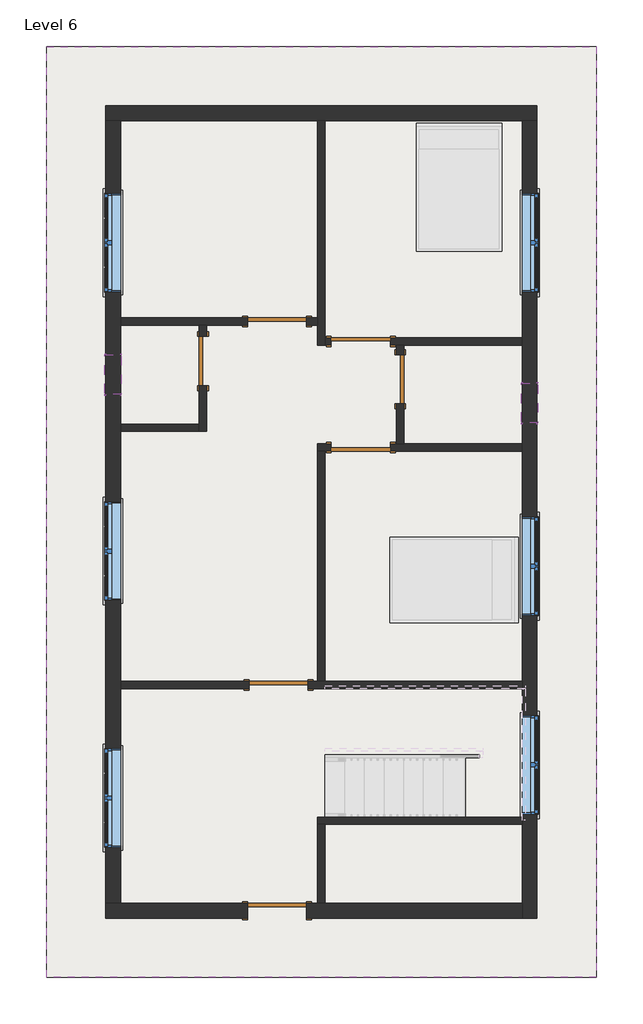
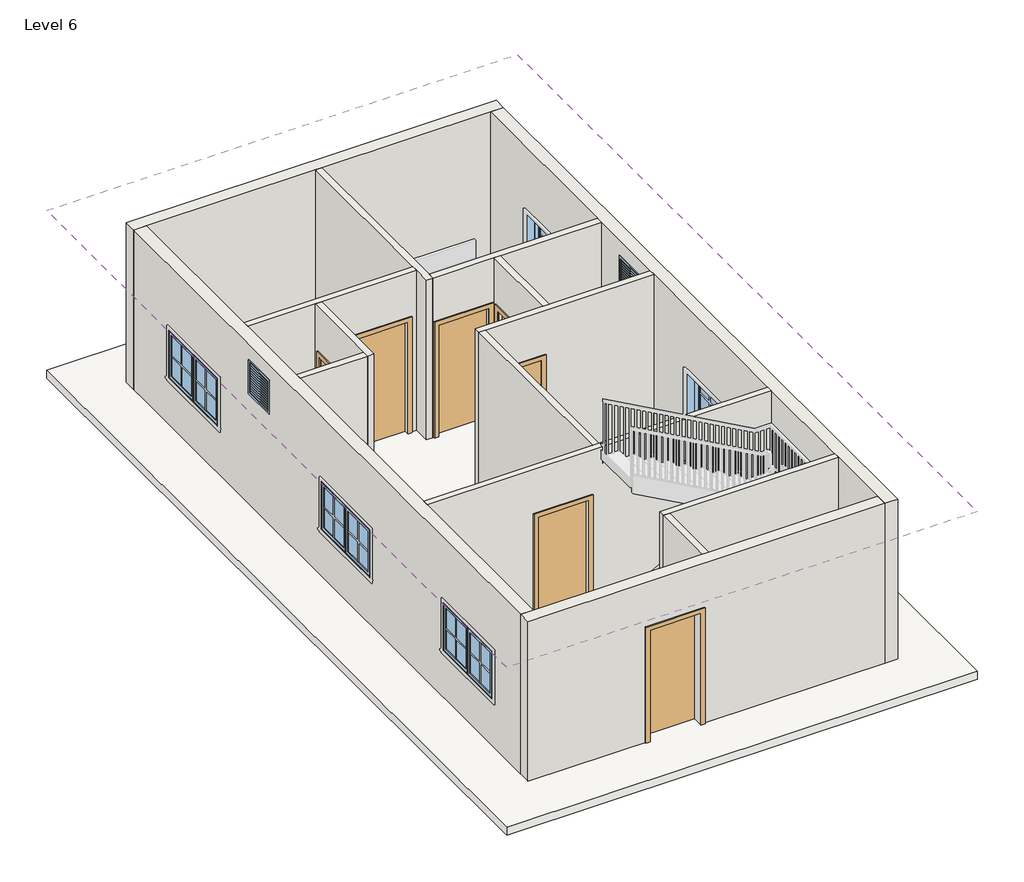
# One storey, part 1 of 3: 15 walls, 8 windows, 7 doors, 2 roofs.
"""IFC4 building model written with IfcOpenShell, lengths in millimetres."""

from ifc_helpers import new_model, si_unit, frame, origin, place, context, project, spatial, polyline, outline, extrude, faceted_brep, transform, mapped, element, save
from components import door_78caadf7, door_214872d5, single_flush_door_3_e5f9f3c4, single_flush_door_3_305aa2a5, single_flush_door_3_0ca8825f, window_casement_double_win_5_c1d95f0f, window_f2d8fef0

model = new_model("IFC4")

# Units and contexts
model_context = context("Model", 3, world=origin())
ifc_project = project(units=[si_unit("LENGTHUNIT", "METRE", prefix="MILLI")], contexts=[model_context])

# Site, building, storey
site = spatial("IfcSite", under=ifc_project)
building = spatial("IfcBuilding", under=site)
storey = spatial("IfcBuildingStorey", under=building, Name="Level 6", Elevation=15849.6)

# Doors
placement = place(None, origin())
door_shape = door_78caadf7(model_context)
element("IfcDoor", 1, ObjectType="Single-Flush : 2'6\"", at=placement, inside=storey, context=model_context, shape_type="MappedRepresentation", body=[
    mapped(door_shape, transform((-35.92188, 1946.24131, 15849.6), x_axis=(0.0, 1.0, 0.0), y_axis=(-1.0, 0.0, 0.0), z_axis=(0.0, 0.0, 1.0))),
])
door_2_shape = door_214872d5(model_context)
element("IfcDoor", 2, ObjectType="Single-Flush : 2'6\"", at=placement, inside=storey, context=model_context, shape_type="MappedRepresentation", body=[
    mapped(door_2_shape, transform((-3083.92188, 2225.64131, 15849.6), x_axis=(0.0, 1.0, 0.0), y_axis=(-1.0, 0.0, 0.0), z_axis=(0.0, 0.0, 1.0))),
])
single_flush_door_3_shape = single_flush_door_3_e5f9f3c4(model_context)
element("IfcDoor", 3, ObjectType="Single-Flush : DOOR 3'", at=placement, inside=storey, context=model_context, shape_type="MappedRepresentation", body=[
    mapped(single_flush_door_3_shape, transform((-1940.92188, 2835.24131, 15849.6), x_axis=(1.0, 0.0, 0.0), y_axis=(0.0, 1.0, 0.0), z_axis=(0.0, 0.0, 1.0))),
])
element("IfcDoor", 4, ObjectType="Single-Flush : DOOR 3'", at=placement, inside=storey, context=model_context, shape_type="MappedRepresentation", body=[
    mapped(single_flush_door_3_shape, transform((-645.52188, 892.14131, 15849.6), x_axis=(-1.0, 0.0, 0.0), y_axis=(0.0, -1.0, 0.0), z_axis=(0.0, 0.0, 1.0))),
])
element("IfcDoor", 5, ObjectType="Single-Flush : DOOR 3'", at=placement, inside=storey, context=model_context, shape_type="MappedRepresentation", body=[
    mapped(single_flush_door_3_shape, transform((-1915.52188, -2778.15869, 15849.6), x_axis=(1.0, 0.0, 0.0), y_axis=(0.0, 1.0, 0.0), z_axis=(0.0, 0.0, 1.0))),
])
single_flush_door_3_2_shape = single_flush_door_3_305aa2a5(model_context)
element("IfcDoor", 6, ObjectType="Single-Flush : DOOR 3'", at=placement, inside=storey, context=model_context, shape_type="MappedRepresentation", body=[
    mapped(single_flush_door_3_2_shape, transform((-645.52188, 2530.44131, 15849.6), x_axis=(-1.0, 0.0, 0.0), y_axis=(0.0, -1.0, 0.0), z_axis=(0.0, 0.0, 1.0))),
])
single_flush_door_3_3_shape = single_flush_door_3_0ca8825f(model_context)
element("IfcDoor", 7, ObjectType="Single-Flush : DOOR 3'", at=placement, inside=storey, context=model_context, shape_type="MappedRepresentation", body=[
    mapped(single_flush_door_3_3_shape, transform((-1940.92188, -6264.30869, 15849.6), x_axis=(1.0, 0.0, 0.0), y_axis=(0.0, 1.0, 0.0), z_axis=(0.0, 0.0, 1.0))),
])

# Roofs
element("IfcRoof", 8, ObjectType="ROOF 6\"", at=placement, inside=storey, context=model_context, shape_type="SweptSolid", body=[
    extrude(outline(polyline([(-5503.27188, 7083.39131), (2993.02812, 7083.39131), (2993.02812, -7293.00869), (-5503.27188, -7293.00869), (-5503.27188, 7083.39131)])), frame((0.0, 0.0, 15697.2), z_axis=(0.0, 0.0, 1.0), x_axis=(1.0, 0.0, 0.0)), (0.0, 0.0, 1.0), 152.4),
])
element("IfcRoof", 9, ObjectType="ROOF 6\"", at=placement, inside=storey, context=model_context, shape_type="SweptSolid", body=[
    extrude(outline(polyline([(-5503.27188, 7083.39131), (2993.02812, 7083.39131), (2993.02812, -7293.00869), (-5503.27188, -7293.00869), (-5503.27188, 7083.39131)])), frame((0.0, 0.0, 18897.6), z_axis=(0.0, 0.0, 1.0), x_axis=(1.0, 0.0, 0.0)), (0.0, 0.0, 1.0), 152.4),
])

# Walls
element("IfcWall", 10, ObjectType="WALL 4.5'", at=placement, inside=storey, context=model_context, shape_type="Brep", body=[
    faceted_brep([(-1312.27188, 5940.39131, 15849.6), (-1312.27188, 2892.39131, 15849.6), (-1312.27188, 2778.09131, 15849.6), (-1312.27188, 2473.29131, 15849.6), (-1312.27188, 2473.29131, 18897.6), (-1312.27188, 2778.09131, 18897.6), (-1312.27188, 2892.39131, 18897.6), (-1312.27188, 5940.39131, 18897.6), (-1197.97188, 5940.39131, 15849.6), (-1197.97188, 5940.39131, 18897.6), (-1197.97188, 2587.59131, 18897.6), (-1197.97188, 2473.29131, 18897.6), (-1197.97188, 2473.29131, 15849.6), (-1197.97188, 2587.59131, 15849.6)], [[[0, 1, 2, 3, 4, 5, 6, 7]], [[8, 9, 10, 11, 12, 13]], [[3, 2, 1, 0, 8, 13, 12]], [[0, 7, 9, 8]], [[4, 3, 12, 11]], [[7, 6, 5, 4, 11, 10, 9]]]),
])
element("IfcWall", 11, ObjectType="WALL 4.5'", at=placement, inside=storey, context=model_context, shape_type="Brep", body=[
    faceted_brep([(-1197.97188, 2473.29131, 15849.6), (-1102.72188, 2473.29131, 15849.6), (-1102.72188, 2473.29131, 17983.2), (-188.32188, 2473.29131, 17983.2), (-188.32188, 2473.29131, 15849.6), (-93.07188, 2473.29131, 15849.6), (21.22812, 2473.29131, 15849.6), (1850.02812, 2473.29131, 15849.6), (1850.02812, 2473.29131, 18897.6), (21.22812, 2473.29131, 18897.6), (-93.07188, 2473.29131, 18897.6), (-1197.97188, 2473.29131, 18897.6), (-1102.72188, 2587.59131, 17983.2), (-1102.72188, 2587.59131, 15849.6), (-1197.97188, 2587.59131, 15849.6), (-1197.97188, 2587.59131, 18897.6), (1850.02812, 2587.59131, 18897.6), (1850.02812, 2587.59131, 15849.6), (-188.32188, 2587.59131, 15849.6), (-188.32188, 2587.59131, 17983.2)], [[[0, 1, 2, 3, 4, 5, 6, 7, 8, 9, 10, 11]], [[12, 13, 14, 15, 16, 17, 18, 19]], [[18, 17, 7, 6, 5, 4]], [[14, 13, 1, 0]], [[0, 11, 15, 14]], [[8, 7, 17, 16]], [[2, 1, 13, 12]], [[3, 2, 12, 19]], [[4, 3, 19, 18]], [[11, 10, 9, 8, 16, 15]]]),
])
element("IfcWall", 12, ObjectType="WALL 4.5'", at=placement, inside=storey, context=model_context, shape_type="Brep", body=[
    faceted_brep([(-1312.27188, 2892.39131, 15849.6), (-1483.72188, 2892.39131, 15849.6), (-1483.72188, 2892.39131, 17983.2), (-2398.12188, 2892.39131, 17983.2), (-2398.12188, 2892.39131, 15849.6), (-4360.27188, 2892.39131, 15849.6), (-4360.27188, 2892.39131, 18897.6), (-1312.27188, 2892.39131, 18897.6), (-1483.72188, 2778.09131, 17983.2), (-1483.72188, 2778.09131, 15849.6), (-1312.27188, 2778.09131, 15849.6), (-1312.27188, 2778.09131, 18897.6), (-3026.77188, 2778.09131, 18897.6), (-3141.07188, 2778.09131, 18897.6), (-4360.27188, 2778.09131, 18897.6), (-4360.27188, 2778.09131, 15849.6), (-3141.07188, 2778.09131, 15849.6), (-3026.77188, 2778.09131, 15849.6), (-2398.12188, 2778.09131, 15849.6), (-2398.12188, 2778.09131, 17983.2)], [[[0, 1, 2, 3, 4, 5, 6, 7]], [[8, 9, 10, 11, 12, 13, 14, 15, 16, 17, 18, 19]], [[10, 9, 1, 0]], [[18, 17, 16, 15, 5, 4]], [[6, 5, 15, 14]], [[0, 7, 11, 10]], [[2, 1, 9, 8]], [[3, 2, 8, 19]], [[4, 3, 19, 18]], [[7, 6, 14, 13, 12, 11]]]),
])
element("IfcWall", 13, ObjectType="WALL 4.5'", at=placement, inside=storey, context=model_context, shape_type="Brep", body=[
    faceted_brep([(-3141.07188, 2778.09131, 15849.6), (-3141.07188, 2606.64131, 15849.6), (-3141.07188, 2606.64131, 17983.2), (-3141.07188, 1844.64131, 17983.2), (-3141.07188, 1844.64131, 15849.6), (-3141.07188, 1254.09131, 15849.6), (-3141.07188, 1139.79131, 15849.6), (-3141.07188, 1139.79131, 18897.6), (-3141.07188, 1254.09131, 18897.6), (-3141.07188, 2778.09131, 18897.6), (-3026.77188, 2606.64131, 17983.2), (-3026.77188, 2606.64131, 15849.6), (-3026.77188, 2778.09131, 15849.6), (-3026.77188, 2778.09131, 18897.6), (-3026.77188, 1139.79131, 18897.6), (-3026.77188, 1139.79131, 15849.6), (-3026.77188, 1844.64131, 15849.6), (-3026.77188, 1844.64131, 17983.2)], [[[0, 1, 2, 3, 4, 5, 6, 7, 8, 9]], [[10, 11, 12, 13, 14, 15, 16, 17]], [[16, 15, 6, 5, 4]], [[12, 11, 1, 0]], [[0, 9, 13, 12]], [[7, 6, 15, 14]], [[2, 1, 11, 10]], [[3, 2, 10, 17]], [[4, 3, 17, 16]], [[9, 8, 7, 14, 13]]]),
])
element("IfcWall", 14, ObjectType="WALL 4.5'", at=placement, inside=storey, context=model_context, shape_type="SweptSolid", body=[
    extrude(outline(polyline([(-4360.27188, 1254.09131), (-3141.07188, 1254.09131), (-3141.07188, 1139.79131), (-4360.27188, 1139.79131), (-4360.27188, 1254.09131)])), frame((0.0, 0.0, 15849.6), z_axis=(0.0, 0.0, 1.0), x_axis=(1.0, 0.0, 0.0)), (0.0, 0.0, 1.0), 3048.0),
])
element("IfcWall", 15, ObjectType="WALL 4.5'", at=placement, inside=storey, context=model_context, shape_type="SweptSolid", body=[
    extrude(outline(polyline([(2473.29131, 15849.6), (2327.24131, 15849.6), (2327.24131, 17983.2), (1565.24131, 17983.2), (1565.24131, 15849.6), (949.29131, 15849.6), (949.29131, 18897.6), (2473.29131, 18897.6), (2473.29131, 15849.6)])), frame((-93.07188, 0.0, 0.0), z_axis=(1.0, 0.0, 0.0), x_axis=(0.0, 1.0, 0.0)), (0.0, 0.0, 1.0), 114.3),
])
element("IfcWall", 16, ObjectType="WALL 4.5'", at=placement, inside=storey, context=model_context, shape_type="Brep", body=[
    faceted_brep([(-1102.72188, 949.29131, 17983.2), (-1102.72188, 949.29131, 15849.6), (-1312.27188, 949.29131, 15849.6), (-1312.27188, 949.29131, 18897.6), (-93.07188, 949.29131, 18897.6), (21.22812, 949.29131, 18897.6), (1850.02812, 949.29131, 18897.6), (1850.02812, 949.29131, 15849.6), (21.22812, 949.29131, 15849.6), (-93.07188, 949.29131, 15849.6), (-188.32188, 949.29131, 15849.6), (-188.32188, 949.29131, 17983.2), (-1312.27188, 834.99131, 15849.6), (-1197.97188, 834.99131, 15849.6), (-1102.72188, 834.99131, 15849.6), (-1102.72188, 834.99131, 17983.2), (-188.32188, 834.99131, 17983.2), (-188.32188, 834.99131, 15849.6), (1850.02812, 834.99131, 15849.6), (1850.02812, 834.99131, 18897.6), (-1197.97188, 834.99131, 18897.6), (-1312.27188, 834.99131, 18897.6)], [[[0, 1, 2, 3, 4, 5, 6, 7, 8, 9, 10, 11]], [[12, 13, 14, 15, 16, 17, 18, 19, 20, 21]], [[2, 1, 14, 13, 12]], [[10, 9, 8, 7, 18, 17]], [[7, 6, 19, 18]], [[3, 2, 12, 21]], [[15, 14, 1, 0]], [[16, 15, 0, 11]], [[17, 16, 11, 10]], [[6, 5, 4, 3, 21, 20, 19]]]),
])
element("IfcWall", 17, ObjectType="WALL 4.5'", at=placement, inside=storey, context=model_context, shape_type="SweptSolid", body=[
    extrude(outline(polyline([(-1312.27188, -2721.00869), (-1312.27188, 834.99131), (-1197.97188, 834.99131), (-1197.97188, -2721.00869), (-1312.27188, -2721.00869)])), frame((0.0, 0.0, 15849.6), z_axis=(0.0, 0.0, 1.0), x_axis=(1.0, 0.0, 0.0)), (0.0, 0.0, 1.0), 3048.0),
])
element("IfcWall", 18, ObjectType="WALL 4.5'", at=placement, inside=storey, context=model_context, shape_type="Brep", body=[
    faceted_brep([(1850.02812, -2721.00869, 15849.6), (-1197.97188, -2721.00869, 15849.6), (-1312.27188, -2721.00869, 15849.6), (-1458.32188, -2721.00869, 15849.6), (-1458.32188, -2721.00869, 17983.2), (-2372.72188, -2721.00869, 17983.2), (-2372.72188, -2721.00869, 15849.6), (-4360.27188, -2721.00869, 15849.6), (-4360.27188, -2721.00869, 18897.6), (-1312.27188, -2721.00869, 18897.6), (-1197.97188, -2721.00869, 18897.6), (1850.02812, -2721.00869, 18897.6), (-1458.32188, -2835.30869, 17983.2), (-1458.32188, -2835.30869, 15849.6), (1850.02812, -2835.30869, 15849.6), (1850.02812, -2835.30869, 18897.6), (-4360.27188, -2835.30869, 18897.6), (-4360.27188, -2835.30869, 15849.6), (-2372.72188, -2835.30869, 15849.6), (-2372.72188, -2835.30869, 17983.2)], [[[0, 1, 2, 3, 4, 5, 6, 7, 8, 9, 10, 11]], [[12, 13, 14, 15, 16, 17, 18, 19]], [[18, 17, 7, 6]], [[14, 13, 3, 2, 1, 0]], [[0, 11, 15, 14]], [[8, 7, 17, 16]], [[4, 3, 13, 12]], [[5, 4, 12, 19]], [[6, 5, 19, 18]], [[11, 10, 9, 8, 16, 15]]]),
])
element("IfcWall", 19, ObjectType="WALL 4.5'", at=placement, inside=storey, context=model_context, shape_type="Brep", body=[
    faceted_brep([(1850.02812, -4816.50869, 15849.6), (-1312.27188, -4816.50869, 15849.6), (-1312.27188, -4816.50869, 18897.6), (1850.02812, -4816.50869, 18897.6), (1850.02812, -4930.80869, 15849.6), (1850.02812, -4930.80869, 18897.6), (-1197.97188, -4930.80869, 18897.6), (-1312.27188, -4930.80869, 18897.6), (-1312.27188, -4930.80869, 15849.6), (-1197.97188, -4930.80869, 15849.6)], [[[0, 1, 2, 3]], [[4, 5, 6, 7, 8, 9]], [[1, 0, 4, 9, 8]], [[0, 3, 5, 4]], [[2, 1, 8, 7]], [[3, 2, 7, 6, 5]]]),
])
element("IfcWall", 20, ObjectType="WALL 4.5'", at=placement, inside=storey, context=model_context, shape_type="SweptSolid", body=[
    extrude(outline(polyline([(-1312.27188, -6150.00869), (-1312.27188, -4930.80869), (-1197.97188, -4930.80869), (-1197.97188, -6150.00869), (-1312.27188, -6150.00869)])), frame((0.0, 0.0, 15849.6), z_axis=(0.0, 0.0, 1.0), x_axis=(1.0, 0.0, 0.0)), (0.0, 0.0, 1.0), 3048.0),
])
element("IfcWall", 21, ObjectType="WALL 9\"", at=placement, inside=storey, context=model_context, shape_type="Brep", body=[
    faceted_brep([(-4588.87188, 5940.39131, 15849.6), (-4360.27188, 5940.39131, 15849.6), (-1312.27188, 5940.39131, 15849.6), (-1197.97188, 5940.39131, 15849.6), (1850.02812, 5940.39131, 15849.6), (2078.62812, 5940.39131, 15849.6), (2078.62812, 5940.39131, 18897.6), (1850.02812, 5940.39131, 18897.6), (-1197.97188, 5940.39131, 18897.6), (-1312.27188, 5940.39131, 18897.6), (-4360.27188, 5940.39131, 18897.6), (-4588.87188, 5940.39131, 18897.6), (-4588.87188, 6168.99131, 15849.6), (-4588.87188, 6168.99131, 18897.6), (2078.62812, 6168.99131, 18897.6), (2078.62812, 6168.99131, 15849.6)], [[[0, 1, 2, 3, 4, 5, 6, 7, 8, 9, 10, 11]], [[12, 13, 14, 15]], [[5, 4, 3, 2, 1, 0, 12, 15]], [[6, 5, 15, 14]], [[0, 11, 13, 12]], [[11, 10, 9, 8, 7, 6, 14, 13]]]),
])
element("IfcWall", 22, ObjectType="WALL 9\"", at=placement, inside=storey, context=model_context, shape_type="Brep", body=[
    faceted_brep([(1850.02812, 5940.39131, 15849.6), (1850.02812, 2587.59131, 15849.6), (1850.02812, 2473.29131, 15849.6), (1850.02812, 949.29131, 15849.6), (1850.02812, 834.99131, 15849.6), (1850.02812, -2721.00869, 15849.6), (1850.02812, -2835.30869, 15849.6), (1850.02812, -4816.50869, 15849.6), (1850.02812, -4930.80869, 15849.6), (1850.02812, -6150.00869, 15849.6), (1850.02812, -6378.60869, 15849.6), (1850.02812, -6378.60869, 18897.6), (1850.02812, -6150.00869, 18897.6), (1850.02812, -4930.80869, 18897.6), (1850.02812, -4816.50869, 18897.6), (1850.02812, -2835.30869, 18897.6), (1850.02812, -2721.00869, 18897.6), (1850.02812, 834.99131, 18897.6), (1850.02812, 949.29131, 18897.6), (1850.02812, 2473.29131, 18897.6), (1850.02812, 2587.59131, 18897.6), (1850.02812, 5940.39131, 18897.6), (1850.02812, -4772.05869, 17678.4), (1850.02812, -4772.05869, 16764.0), (1850.02812, -3248.05869, 16764.0), (1850.02812, -3248.05869, 17678.4), (1850.02812, 3292.44131, 17678.4), (1850.02812, 3292.44131, 16764.0), (1850.02812, 4816.44131, 16764.0), (1850.02812, 4816.44131, 17678.4), (1850.02812, -1705.00869, 17678.4), (1850.02812, -1705.00869, 16764.0), (1850.02812, -181.00869, 16764.0), (1850.02812, -181.00869, 17678.4), (1850.02812, 1273.14131, 18592.8), (1850.02812, 1273.14131, 17983.2), (1850.02812, 1882.74131, 17983.2), (1850.02812, 1882.74131, 18592.8), (2078.62812, 5940.39131, 15849.6), (2078.62812, 5940.39131, 18897.6), (2078.62812, -6378.60869, 18897.6), (2078.62812, -6378.60869, 15849.6), (2078.62812, -4772.05869, 17678.4), (2078.62812, -3248.05869, 17678.4), (2078.62812, -3248.05869, 16764.0), (2078.62812, -4772.05869, 16764.0), (2078.62812, 3292.44131, 17678.4), (2078.62812, 4816.44131, 17678.4), (2078.62812, 4816.44131, 16764.0), (2078.62812, 3292.44131, 16764.0), (2078.62812, -1705.00869, 17678.4), (2078.62812, -181.00869, 17678.4), (2078.62812, -181.00869, 16764.0), (2078.62812, -1705.00869, 16764.0), (2078.62812, 1273.14131, 18592.8), (2078.62812, 1882.74131, 18592.8), (2078.62812, 1882.74131, 17983.2), (2078.62812, 1273.14131, 17983.2)], [[[0, 1, 2, 3, 4, 5, 6, 7, 8, 9, 10, 11, 12, 13, 14, 15, 16, 17, 18, 19, 20, 21], [22, 23, 24, 25], [26, 27, 28, 29], [30, 31, 32, 33], [34, 35, 36, 37]], [[38, 39, 40, 41], [42, 43, 44, 45], [46, 47, 48, 49], [50, 51, 52, 53], [54, 55, 56, 57]], [[10, 9, 8, 7, 6, 5, 4, 3, 2, 1, 0, 38, 41]], [[0, 21, 39, 38]], [[11, 10, 41, 40]], [[23, 22, 42, 45]], [[24, 23, 45, 44]], [[25, 24, 44, 43]], [[22, 25, 43, 42]], [[27, 26, 46, 49]], [[28, 27, 49, 48]], [[29, 28, 48, 47]], [[26, 29, 47, 46]], [[31, 30, 50, 53]], [[32, 31, 53, 52]], [[33, 32, 52, 51]], [[30, 33, 51, 50]], [[35, 34, 54, 57]], [[36, 35, 57, 56]], [[37, 36, 56, 55]], [[34, 37, 55, 54]], [[21, 20, 19, 18, 17, 16, 15, 14, 13, 12, 11, 40, 39]]]),
])
element("IfcWall", 23, ObjectType="WALL 9\"", at=placement, inside=storey, context=model_context, shape_type="Brep", body=[
    faceted_brep([(1850.02812, -6150.00869, 15849.6), (-1197.97188, -6150.00869, 15849.6), (-1312.27188, -6150.00869, 15849.6), (-1483.72188, -6150.00869, 15849.6), (-1483.72188, -6150.00869, 17983.2), (-2398.12188, -6150.00869, 17983.2), (-2398.12188, -6150.00869, 15849.6), (-4360.27188, -6150.00869, 15849.6), (-4588.87188, -6150.00869, 15849.6), (-4588.87188, -6150.00869, 18897.6), (-4360.27188, -6150.00869, 18897.6), (-1312.27188, -6150.00869, 18897.6), (-1197.97188, -6150.00869, 18897.6), (1850.02812, -6150.00869, 18897.6), (-1483.72188, -6378.60869, 17983.2), (-1483.72188, -6378.60869, 15849.6), (1850.02812, -6378.60869, 15849.6), (1850.02812, -6378.60869, 18897.6), (-4588.87188, -6378.60869, 18897.6), (-4588.87188, -6378.60869, 15849.6), (-2398.12188, -6378.60869, 15849.6), (-2398.12188, -6378.60869, 17983.2)], [[[0, 1, 2, 3, 4, 5, 6, 7, 8, 9, 10, 11, 12, 13]], [[14, 15, 16, 17, 18, 19, 20, 21]], [[20, 19, 8, 7, 6]], [[16, 15, 3, 2, 1, 0]], [[0, 13, 17, 16]], [[9, 8, 19, 18]], [[4, 3, 15, 14]], [[5, 4, 14, 21]], [[6, 5, 21, 20]], [[13, 12, 11, 10, 9, 18, 17]]]),
])
element("IfcWall", 24, ObjectType="WALL 9\"", at=placement, inside=storey, context=model_context, shape_type="Brep", body=[
    faceted_brep([(-4360.27188, -6150.00869, 15849.6), (-4360.27188, -2835.30869, 15849.6), (-4360.27188, -2721.00869, 15849.6), (-4360.27188, 1139.79131, 15849.6), (-4360.27188, 1254.09131, 15849.6), (-4360.27188, 2778.09131, 15849.6), (-4360.27188, 2892.39131, 15849.6), (-4360.27188, 5940.39131, 15849.6), (-4360.27188, 5940.39131, 18897.6), (-4360.27188, 2892.39131, 18897.6), (-4360.27188, 2778.09131, 18897.6), (-4360.27188, 1254.09131, 18897.6), (-4360.27188, 1139.79131, 18897.6), (-4360.27188, -2721.00869, 18897.6), (-4360.27188, -2835.30869, 18897.6), (-4360.27188, -6150.00869, 18897.6), (-4360.27188, 4816.44131, 17678.4), (-4360.27188, 4816.44131, 16764.0), (-4360.27188, 3292.44131, 16764.0), (-4360.27188, 3292.44131, 17678.4), (-4360.27188, 53.94131, 17678.4), (-4360.27188, 53.94131, 16764.0), (-4360.27188, -1470.05869, 16764.0), (-4360.27188, -1470.05869, 17678.4), (-4360.27188, -3759.23369, 17678.4), (-4360.27188, -3759.23369, 16764.0), (-4360.27188, -5283.23369, 16764.0), (-4360.27188, -5283.23369, 17678.4), (-4360.27188, 1711.29131, 18592.8), (-4360.27188, 2320.89131, 18592.8), (-4360.27188, 2320.89131, 17983.2), (-4360.27188, 1711.29131, 17983.2), (-4588.87188, -6150.00869, 15849.6), (-4588.87188, -6150.00869, 18897.6), (-4588.87188, 5940.39131, 18897.6), (-4588.87188, 5940.39131, 15849.6), (-4588.87188, 4816.44131, 17678.4), (-4588.87188, 3292.44131, 17678.4), (-4588.87188, 3292.44131, 16764.0), (-4588.87188, 4816.44131, 16764.0), (-4588.87188, 53.94131, 17678.4), (-4588.87188, -1470.05869, 17678.4), (-4588.87188, -1470.05869, 16764.0), (-4588.87188, 53.94131, 16764.0), (-4588.87188, -3759.23369, 17678.4), (-4588.87188, -5283.23369, 17678.4), (-4588.87188, -5283.23369, 16764.0), (-4588.87188, -3759.23369, 16764.0), (-4588.87188, 1711.29131, 18592.8), (-4588.87188, 1711.29131, 17983.2), (-4588.87188, 2320.89131, 17983.2), (-4588.87188, 2320.89131, 18592.8)], [[[0, 1, 2, 3, 4, 5, 6, 7, 8, 9, 10, 11, 12, 13, 14, 15], [16, 17, 18, 19], [20, 21, 22, 23], [24, 25, 26, 27], [28, 29, 30, 31]], [[32, 33, 34, 35], [36, 37, 38, 39], [40, 41, 42, 43], [44, 45, 46, 47], [48, 49, 50, 51]], [[7, 6, 5, 4, 3, 2, 1, 0, 32, 35]], [[8, 7, 35, 34]], [[0, 15, 33, 32]], [[17, 16, 36, 39]], [[18, 17, 39, 38]], [[19, 18, 38, 37]], [[16, 19, 37, 36]], [[21, 20, 40, 43]], [[22, 21, 43, 42]], [[23, 22, 42, 41]], [[20, 23, 41, 40]], [[25, 24, 44, 47]], [[26, 25, 47, 46]], [[27, 26, 46, 45]], [[24, 27, 45, 44]], [[49, 48, 28, 31]], [[50, 49, 31, 30]], [[51, 50, 30, 29]], [[48, 51, 29, 28]], [[15, 14, 13, 12, 11, 10, 9, 8, 34, 33]]]),
])

# Windows
window_casement_double_win_5_shape = window_casement_double_win_5_c1d95f0f(model_context)
element("IfcWindow", 25, ObjectType="Window-Casement-Double : WIN 5'", at=placement, inside=storey, context=model_context, shape_type="MappedRepresentation", body=[
    mapped(window_casement_double_win_5_shape, transform((-4474.57188, 4054.44131, 15849.6), x_axis=(0.0, 1.0, 0.0), y_axis=(-1.0, 0.0, 0.0), z_axis=(0.0, 0.0, 1.0))),
])
element("IfcWindow", 26, ObjectType="Window-Casement-Double : WIN 5'", at=placement, inside=storey, context=model_context, shape_type="MappedRepresentation", body=[
    mapped(window_casement_double_win_5_shape, transform((-4474.57188, -708.05869, 15849.6), x_axis=(0.0, 1.0, 0.0), y_axis=(-1.0, 0.0, 0.0), z_axis=(0.0, 0.0, 1.0))),
])
element("IfcWindow", 27, ObjectType="Window-Casement-Double : WIN 5'", at=placement, inside=storey, context=model_context, shape_type="MappedRepresentation", body=[
    mapped(window_casement_double_win_5_shape, transform((-4474.57188, -4521.23369, 15849.6), x_axis=(0.0, 1.0, 0.0), y_axis=(-1.0, 0.0, 0.0), z_axis=(0.0, 0.0, 1.0))),
])
element("IfcWindow", 28, ObjectType="Window-Casement-Double : WIN 5'", at=placement, inside=storey, context=model_context, shape_type="MappedRepresentation", body=[
    mapped(window_casement_double_win_5_shape, transform((1964.32812, -4010.05869, 15849.6), x_axis=(0.0, -1.0, 0.0), y_axis=(1.0, 0.0, 0.0), z_axis=(0.0, 0.0, 1.0))),
])
element("IfcWindow", 29, ObjectType="Window-Casement-Double : WIN 5'", at=placement, inside=storey, context=model_context, shape_type="MappedRepresentation", body=[
    mapped(window_casement_double_win_5_shape, transform((1964.32812, 4054.44131, 15849.6), x_axis=(0.0, -1.0, 0.0), y_axis=(1.0, 0.0, 0.0), z_axis=(0.0, 0.0, 1.0))),
])
element("IfcWindow", 30, ObjectType="Window-Casement-Double : WIN 5'", at=placement, inside=storey, context=model_context, shape_type="MappedRepresentation", body=[
    mapped(window_casement_double_win_5_shape, transform((1964.32812, -943.00869, 15849.6), x_axis=(0.0, -1.0, 0.0), y_axis=(1.0, 0.0, 0.0), z_axis=(0.0, 0.0, 1.0))),
])
window_shape = window_f2d8fef0(model_context)
element("IfcWindow", 31, ObjectType="Window-Louvers : 24\" x 24\"", at=placement, inside=storey, context=model_context, shape_type="MappedRepresentation", body=[
    mapped(window_shape, transform((1957.97812, 1577.94131, 17068.8), x_axis=(0.0, 1.0, 0.0), y_axis=(-1.0, 0.0, 0.0), z_axis=(0.0, 0.0, 1.0))),
])
element("IfcWindow", 32, ObjectType="Window-Louvers : 24\" x 24\"", at=placement, inside=storey, context=model_context, shape_type="MappedRepresentation", body=[
    mapped(window_shape, transform((-4480.92188, 2016.09131, 17068.8), x_axis=(0.0, 1.0, 0.0), y_axis=(-1.0, 0.0, 0.0), z_axis=(0.0, 0.0, 1.0))),
])

save(model, "model.ifc")

# Revit data of these elements
# Type "Single-Flush : 2'6\""
#   Type Mark = "9"
#   Construction Type Id = "MDOOR"
#   Assembly Code = "C1020"
#   Analytic Construction = "Metal"
#   Thickness = 0' - 2"
#   Heat Transfer Coefficient (U) = 0.651978 BTU/(h·ft²·°F)
#   Height = 7' - 0"
#   Trim Projection Ext = 0' - 1"
#   Trim Projection Int = 0' - 1"
#   Trim Width = 0' - 3"
#   Width = 2' - 6"
#   Define Thermal Properties by = 1
#   Door Material = Door - Panel
#   Frame Material = Door - Frame
#   Visual Light Transmittance = 0
#   Solar Heat Gain Coefficient = 0
#   Function = (empty or 0)
#   Wall Closure = (empty or 0)
# Type "Single-Flush : DOOR 3'"
#   Type Mark = "8"
#   Construction Type Id = "MDOOR"
#   Assembly Code = "C1020"
#   Analytic Construction = "Metal"
#   Thickness = 0' - 2"
#   Heat Transfer Coefficient (U) = 0.651978 BTU/(h·ft²·°F)
#   Height = 7' - 0"
#   Trim Projection Ext = 0' - 1"
#   Trim Projection Int = 0' - 1"
#   Trim Width = 0' - 3"
#   Width = 3' - 0"
#   Define Thermal Properties by = 1
#   Door Material = Door - Panel
#   Frame Material = Door - Frame
#   Visual Light Transmittance = 0
#   Solar Heat Gain Coefficient = 0
#   Function = (empty or 0)
#   Wall Closure = (empty or 0)
# Type "ROOF 6\""
#   Assembly Code = "B1020"
#   Layers, outside or top first: 0' - 6" no material (function 1)
# Type "WALL 4.5'"
#   Assembly Code = "B2010"
#   Layers, outside or top first: 0' - 4 1/2" no material (function 1)
# Type "WALL 9\""
#   Assembly Code = "B2010"
#   Layers, outside or top first: 0' - 9" no material (function 1)
# Type "Window-Casement-Double : WIN 5'"
#   Type Mark = "18"
#   Fire Rating = "0.5h"
#   Assembly Code = "B2020100"
#   Analytic Construction = "Double glazing - domestic"
#   Frame Extension [instance default] = 0' - 0 1/4"
#   Window Inset [instance default] = 0' - 0"
#   Wall Thickness [instance default] = 0' - 6"
#   Interior Wall Closure [instance default] = 0' - 2 1/4"
#   Half Width = 2' - 6"
#   Visual Light Transmittance = 0.81
#   Thermal Resistance (R) = 1.8146 (h·ft²·°F)/BTU
#   Solar Heat Gain Coefficient = 0.76
#   Rough Width = 5' - 0 1/2"
#   Rough Height = 3' - 0 1/2"
#   Height = 3' - 0"
#   Heat Transfer Coefficient (U) = 0.5511 BTU/(h·ft²·°F)
#   Exterior Wall Closure [instance default] = 0' - 1 1/4"
#   Extension Jamb [instance default] = 0' - 2 1/4"
#   Default Sill Height = 3' - 0"
#   Width = 5' - 0"
#   Muntin Visibility = yes
#   Interior Trim Visibility [instance default] = yes
#   Exterior Trim Visibility [instance default] = yes
#   Extension Jamb Visibility [instance default] = yes
#   Interior Trim Material = Wood - Stained
#   Muntin Pattern = Muntin Pattern_2x2 : Muntin Pattern_2x2
#   Interior Trim = Trim-Window-Interior-Flat : Picture Frame
#   Interior Frame Material = Wood - Stained
#   Glass Panel Material = Glass
#   Exterior Trim Material = Clad - White
#   Exterior Trim = Trim-Window-Exterior-Flat : with Sill
#   Exterior Frame Material = Clad - White
#   Wall Closure = (empty or 0)
# Type "Window-Louvers : 24\" x 24\""
#   Type Mark = "19"
#   Construction Type Id = "GSP4R"
#   Assembly Code = "B20"
#   Analytic Construction = "1/8 in Pilkington single glazing"
#   Visual Light Transmittance = 0.9
#   Thermal Resistance (R) = 1.53941 (h·ft²·°F)/BTU
#   Solar Heat Gain Coefficient = 0.78
#   Max Height = 1' - 11.74264"
#   Height = 2' - 0"
#   Heat Transfer Coefficient (U) = 0.6496 BTU/(h·ft²·°F)
#   Blade Width [instance default] = 1' - 10 1/2"
#   Blade Vertical Thickness = 0' - 0.35355"
#   Blade Thickness = 0' - 0 1/4"
#   Blade Spacing = 0' - 1 1/2"
#   Blade Height = 0' - 1.85355"
#   Blade Depth = 0' - 3"
#   Blade Angle = 45.00°
#   Default Sill Height = 3' - 0"
#   Trim Projection_Exterior = 0' - 0 1/2"
#   Trim Projection_Interior = 0' - 0 1/2"
#   Trim Width_Exterior = 0' - 1 1/2"
#   Trim Width_Interior = 0' - 1 1/2"
#   Width = 2' - 0"
#   Max Blade Count = 12
#   Define Thermal Properties by = 1
#   Blade Count = 12
#   Frame Material = Birch
#   Louver Material = Birch
#   Trim Exterior Material = Birch
#   Trim Interior Material = Birch
#   Wall Closure = (empty or 0)
# Elements 1, 2 (IfcDoor, "Single-Flush : 2'6\"")
#   Phase Created = New Construction
#   Materials on its faces: "Door - Frame", "Door - Panel"
# Elements 3, 4, 5, 6, 7 (IfcDoor, "Single-Flush : DOOR 3'")
#   Phase Created = New Construction
#   Materials on its faces: "Door - Frame", "Door - Panel"
# Element 8 (IfcRoof, "ROOF 6\"")
#   built-in parameter 1001705 = 52 (stored number, unit not read)
#   built-in parameter 1001701 = -0.5 (stored number, unit not read)
#   built-in parameter 1001710 = 33615
#   Phase Created = New Construction
#   Materials on its faces: "Parking Stripe", "Default Roof", "Wood - Stained"
# Element 9 (IfcRoof, "ROOF 6\"")
#   built-in parameter 1001705 = 62.5 (stored number, unit not read)
#   built-in parameter 1001701 = 10 (stored number, unit not read)
#   built-in parameter 1001710 = 33615
#   Phase Created = New Construction
#   Materials on its faces: "Parking Stripe", "Default Roof", "Wood - Stained"
# Elements 10, 11, 12, 13, 14, 15, 16, 17, 18, 19, 20 (IfcWall, "WALL 4.5'")
#   Top Offset = 0' - 0"
#   Base Offset = 0' - 0"
#   Unconnected Height = 10' - 0"
#   wall height = 10' - 0"
#   Phase Created = New Construction
#   Base Constraint = Level 6
#   Materials on its faces: "Default Wall"
# Elements 21, 22, 23, 24 (IfcWall, "WALL 9\"")
#   Top Offset = 0' - 0"
#   Base Offset = 0' - 0"
#   Unconnected Height = 10' - 0"
#   wall height = 10' - 0"
#   Phase Created = New Construction
#   Base Constraint = Level 6
#   Materials on its faces: "Default Wall", "Copper"
# Element 25 (IfcWindow, "Window-Casement-Double : WIN 5'")
#   Mark = "41"
#   Window Inset = 0' - 0"
#   Interior Wall Closure = 0' - 2 1/4"
#   Frame Extension = 0' - 0 1/4"
#   Exterior Wall Closure = 0' - 1 1/4"
#   Interior Trim Visibility = yes
#   Exterior Trim Visibility = yes
#   Phase Created = New Construction
#   Materials on its faces: "Wood - Stained", "Glass", "Clad - White"
# Element 26 (IfcWindow, "Window-Casement-Double : WIN 5'")
#   Mark = "42"
#   Window Inset = 0' - 0"
#   Interior Wall Closure = 0' - 2 1/4"
#   Frame Extension = 0' - 0 1/4"
#   Exterior Wall Closure = 0' - 1 1/4"
#   Interior Trim Visibility = yes
#   Exterior Trim Visibility = yes
#   Phase Created = New Construction
#   Materials on its faces: "Wood - Stained", "Glass", "Clad - White"
# Element 27 (IfcWindow, "Window-Casement-Double : WIN 5'")
#   Mark = "43"
#   Window Inset = 0' - 0"
#   Interior Wall Closure = 0' - 2 1/4"
#   Frame Extension = 0' - 0 1/4"
#   Exterior Wall Closure = 0' - 1 1/4"
#   Interior Trim Visibility = yes
#   Exterior Trim Visibility = yes
#   Phase Created = New Construction
#   Materials on its faces: "Wood - Stained", "Glass", "Clad - White"
# Element 28 (IfcWindow, "Window-Casement-Double : WIN 5'")
#   Mark = "44"
#   Window Inset = 0' - 0"
#   Interior Wall Closure = 0' - 2 1/4"
#   Frame Extension = 0' - 0 1/4"
#   Exterior Wall Closure = 0' - 1 1/4"
#   Interior Trim Visibility = yes
#   Exterior Trim Visibility = yes
#   Phase Created = New Construction
#   Materials on its faces: "Wood - Stained", "Glass", "Clad - White"
# Element 29 (IfcWindow, "Window-Casement-Double : WIN 5'")
#   Mark = "45"
#   Window Inset = 0' - 0"
#   Interior Wall Closure = 0' - 2 1/4"
#   Frame Extension = 0' - 0 1/4"
#   Exterior Wall Closure = 0' - 1 1/4"
#   Interior Trim Visibility = yes
#   Exterior Trim Visibility = yes
#   Phase Created = New Construction
#   Materials on its faces: "Wood - Stained", "Glass", "Clad - White"
# Element 30 (IfcWindow, "Window-Casement-Double : WIN 5'")
#   Mark = "46"
#   Window Inset = 0' - 0"
#   Interior Wall Closure = 0' - 2 1/4"
#   Frame Extension = 0' - 0 1/4"
#   Exterior Wall Closure = 0' - 1 1/4"
#   Interior Trim Visibility = yes
#   Exterior Trim Visibility = yes
#   Phase Created = New Construction
#   Materials on its faces: "Wood - Stained", "Glass", "Clad - White"
# Element 31 (IfcWindow, "Window-Louvers : 24\" x 24\"")
#   Mark = "47"
#   Blade Width = 1' - 10 1/2"
#   Phase Created = New Construction
#   Materials on its faces: "Birch"
# Element 32 (IfcWindow, "Window-Louvers : 24\" x 24\"")
#   Mark = "48"
#   Blade Width = 1' - 10 1/2"
#   Phase Created = New Construction
#   Materials on its faces: "Birch"
# Materials
#   "Door - Panel": class "Wood", colour RGB 210 159 95, transparency 0, Cost = 0
#   "Door - Frame": colour RGB 118 70 51, transparency 0, Cost = 0
#   "Wood - Stained": class "Wood", colour RGB 224 178 126, transparency 0, Cost = 0
#   "Glass": class "Glass", colour RGB 0 128 192, transparency 0.75, Description = "Soda Lime Glass", Cost = 0
#   "Clad - White": class "Wood", colour RGB 242 242 238, transparency 0, Cost = 0
#   "Birch": class "Wood", colour RGB 224 178 126, transparency 0, Description = "Betula Alleghaniensis", Cost = 0
#   "Parking Stripe": class "Paint", colour RGB 250 250 91, transparency 0, Cost = 0
#   "Default Roof": colour RGB 88 101 114, transparency 0, Cost = 0
#   "Default Wall": colour RGB 128 128 128, transparency 0, Cost = 0
#   "Copper": class "Metal", colour RGB 0 0 0, transparency 0, Description = "Copper, matte finish", Cost = 0
